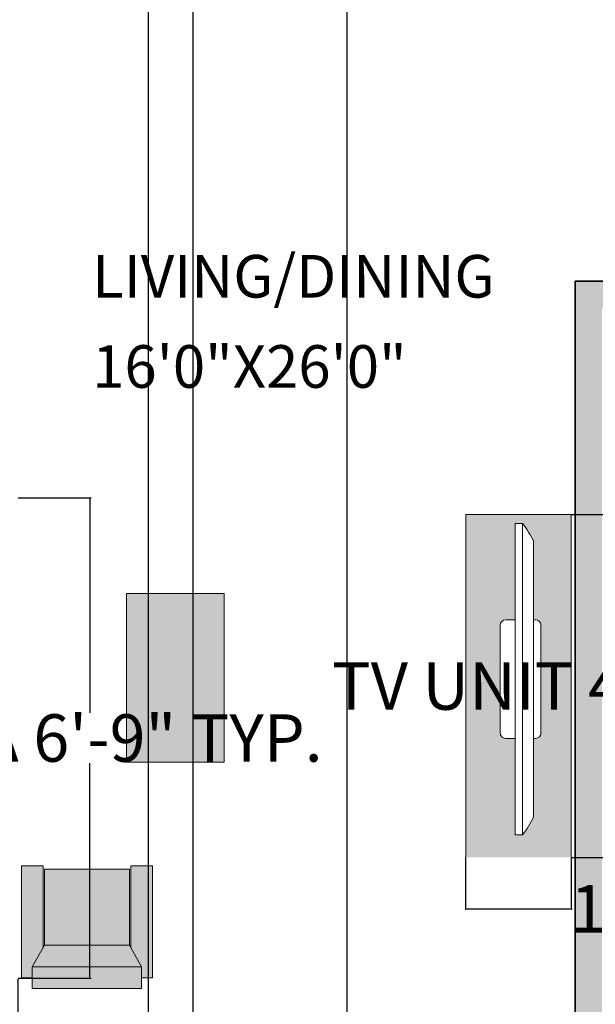
# Model space of a CAD drawing. Units: inches. Extents: x 853 to 1550, y 485 to 1596.
# Tile 6 of 18: x 1170 to 1267, y 867 to 1034. Entities that reach past the tile are written whole.
import ezdxf

# ---------------------------------------------------------------- set-up
doc = ezdxf.new("R2010")
doc.units = ezdxf.units.IN
doc.header["$MEASUREMENT"] = 0
for name, color, linetype, lineweight in [('A-ANNO-DIMS', 2, 'Continuous', 18), ('A-AREA-IDEN', 250, 'Continuous', 18), ('A-WALL-PATT', 250, 'Continuous', 13), ('furniture', 250, 'Continuous', 18), ('walls', 250, 'Continuous', 35)]:
    doc.layers.add(name, color=color, linetype=linetype, lineweight=lineweight)
doc.layers.add('A-FURN-PATT', color=254, linetype='Continuous', lineweight=13, true_color=0xfeeab9)
doc.styles.get("Standard").update_dxf_attribs({"font": 'arial.ttf'})
doc.dimstyles.get("Standard").update_dxf_attribs({"dimtxt": 8, "dimasz": 0.18, "dimexe": 0.18, "dimexo": 0.0625, "dimgap": 0.09, "dimtad": 0, "dimtih": 1, "dimtoh": 1, "dimzin": 0, "dimdsep": 46, "dimlunit": 3, "dimtxsty": 'Standard', "dimcen": 0.09, "dimadec": 0, "dimazin": 0, "dimtfac": 1, "dimtofl": 0, "dimtmove": 0, "dimatfit": 3, "dimfxl": 1, "dimtolj": 1, "dimtzin": 0, "dimarcsym": 0})

# ---------------------------------------------------------------- blocks, each defined once
blk = doc.blocks.new('FABRIC SOFA 1S')
at = {"layer": 'furniture'}
for p, q in [((3, 18.12), (34, 18.12)), ((3, 15.12), (3, 18.12)), ((34, 12.12), (34, 18.12)), ((0, -15.12), (0, 15.12)), ((6, 15.12), (0, 15.12)), ((6, -15.12), (6, 15.12)), ((12, 11.75), (6, 15.12)), ((11.33, 12.12), (34, 12.12)), ((6, -15.12), (12, -11.75)), ((11.33, -12.12), (34, -12.12)), ((34, -12.12), (34, -18.12)), ((6, -15.12), (0, -15.12)), ((3, -18.12), (3, -15.12)), ((3, -18.12), (34, -18.12))]:
    blk.add_line(p, q, dxfattribs=at)
blk.add_lwpolyline([(12, -11.75), (12, 11.75), (33, 11.75), (33, -11.75)], close=True, dxfattribs=at)
blk = doc.blocks.new('PLASMA-LARGE')
at = {"layer": 'furniture'}
for p, q in [((-7.26, 0), (7.26, 0)), ((-18.61, -1), (18.61, -1)), ((-8, -1), (-8, -0.74)), ((8, -1), (8, -0.74)), ((-21, -2.5), (21, -2.5)), ((-21, -2.5), (-21, -3.5)), ((21, -2.5), (21, -3.5)), ((-21, -3.5), (21, -3.5)), ((-8, -3.5), (-8, -4.76)), ((8, -3.5), (8, -4.76)), ((-7.26, -5.5), (7.26, -5.5))]:
    blk.add_line(p, q, dxfattribs=at)
for centre, radius, start, end in [((-7.26, -0.74), 0.744, 90, 180), ((7.26, -0.74), 0.744, 0, 90), ((-13.97, -11.05), 11.07, 114.7602, 129.4175), ((13.97, -11.05), 11.07, 50.5825, 65.2398), ((-7.26, -4.76), 0.744, 180, 270), ((7.26, -4.76), 0.744, 270, 0)]:
    blk.add_arc(centre, radius, start, end, dxfattribs=at)
blk = doc.blocks.new('TV-CONSOLE')
for p, q in [((0, 0), (0, 57.83)), ((0, 57.83), (17.81, 57.83)), ((17.81, 57.83), (17.81, 0))]:
    blk.add_line(p, q)
at = {"xscale": 1.249763490704796, "yscale": 1.249763490704796, "zscale": 1.249763490704796, "rotation": 270}
blk.add_blockref('PLASMA-LARGE', (12.71, 30.08), dxfattribs=at)
blk = doc.blocks.new('*D42')
at = {"layer": 'A-ANNO-DIMS', "color": 0, "lineweight": -2, "transparency": 16777216}
for p, q in [((1293.75, 863.63), (1282.92, 863.63)), ((1283.1, 863.45), (1283.1, 863.3)), ((1293.75, 854.63), (1282.92, 854.63)), ((1283.1, 854.81), (1283.1, 854.95))]:
    blk.add_line(p, q, dxfattribs=at)
at = {"layer": 'A-ANNO-DIMS', "color": 0, "transparency": 16777216}
for points in [[(1283.07, 863.45), (1283.13, 863.45), (1283.1, 863.63)], [(1283.07, 854.81), (1283.13, 854.81), (1283.1, 854.63)]]:
    blk.add_solid(points, dxfattribs=at)
at = {"layer": 'Defpoints', "color": 0, "transparency": 16777216}
for p in [(1283.1, 863.63), (1293.81, 863.63), (1293.81, 854.63)]:
    blk.add_point(p, dxfattribs=at)
at = {"layer": 'A-ANNO-DIMS', "color": 0, "transparency": 16777216, "insert": (1283.1, 859.13), "char_height": 8, "attachment_point": 5}
blk.add_mtext('\\A1;0\'-9" TYP.', dxfattribs=at)
blk = doc.blocks.new('*D45')
at = {"layer": 'A-ANNO-DIMS', "color": 0, "lineweight": -2, "transparency": 16777216}
for p, q in [((1263.33, 950.07), (1272.12, 950.07)), ((1271.94, 949.89), (1271.94, 925.33)), ((1271.94, 892.42), (1271.94, 916.98)), ((1263.33, 892.24), (1272.12, 892.24))]:
    blk.add_line(p, q, dxfattribs=at)
at = {"layer": 'A-ANNO-DIMS', "color": 0, "transparency": 16777216}
for points in [[(1271.91, 949.89), (1271.97, 949.89), (1271.94, 950.07)], [(1271.91, 892.42), (1271.97, 892.42), (1271.94, 892.24)]]:
    blk.add_solid(points, dxfattribs=at)
at = {"layer": 'Defpoints', "color": 0, "transparency": 16777216}
for p in [(1263.27, 950.07), (1271.94, 950.07), (1263.27, 892.24)]:
    blk.add_point(p, dxfattribs=at)
at = {"layer": 'A-ANNO-DIMS', "color": 0, "transparency": 16777216, "insert": (1271.94, 921.15), "char_height": 8, "attachment_point": 5}
blk.add_mtext('\\A1;TV UNIT 4\'-10" TYP.', dxfattribs=at)
blk = doc.blocks.new('*D46')
at = {"layer": 'A-ANNO-DIMS', "color": 0, "lineweight": -2, "transparency": 16777216}
for p, q in [((1245.45, 892.17), (1245.45, 883.38)), ((1263.27, 892.17), (1263.27, 883.38)), ((1245.63, 883.56), (1263.09, 883.56)), ((1263.27, 883.56), (1263.45, 883.56))]:
    blk.add_line(p, q, dxfattribs=at)
at = {"layer": 'A-ANNO-DIMS', "color": 0, "transparency": 16777216}
for points in [[(1245.63, 883.59), (1245.63, 883.53), (1245.45, 883.56)], [(1263.09, 883.59), (1263.09, 883.53), (1263.27, 883.56)]]:
    blk.add_solid(points, dxfattribs=at)
at = {"layer": 'Defpoints', "color": 0, "transparency": 16777216}
for p in [(1245.45, 892.24), (1263.27, 892.24), (1263.27, 883.56)]:
    blk.add_point(p, dxfattribs=at)
at = {"layer": 'A-ANNO-DIMS', "color": 0, "transparency": 16777216, "insert": (1287.54, 883.56), "char_height": 8, "attachment_point": 5}
blk.add_mtext('\\A1;1\'-6" TYP.', dxfattribs=at)
blk = doc.blocks.new('*D49')
at = {"layer": 'A-ANNO-DIMS', "color": 0, "lineweight": -2, "transparency": 16777216}
for p, q in [((1169.96, 952.92), (1182.24, 952.92)), ((1182.06, 952.74), (1182.06, 916.61)), ((1182.06, 872.02), (1182.06, 908.15)), ((1169.96, 871.84), (1182.24, 871.84))]:
    blk.add_line(p, q, dxfattribs=at)
at = {"layer": 'A-ANNO-DIMS', "color": 0, "transparency": 16777216}
for points in [[(1182.03, 952.74), (1182.09, 952.74), (1182.06, 952.92)], [(1182.03, 872.02), (1182.09, 872.02), (1182.06, 871.84)]]:
    blk.add_solid(points, dxfattribs=at)
at = {"layer": 'Defpoints', "color": 0, "transparency": 16777216}
for p in [(1169.9, 952.92), (1182.06, 952.92), (1169.9, 871.84)]:
    blk.add_point(p, dxfattribs=at)
at = {"layer": 'A-ANNO-DIMS', "color": 0, "transparency": 16777216, "insert": (1182.06, 912.38), "char_height": 8, "attachment_point": 5}
blk.add_mtext('\\A1;SOFA 6\'-9" TYP.', dxfattribs=at)
blk = doc.blocks.new('*D50')
at = {"layer": 'A-ANNO-DIMS', "color": 0, "lineweight": -2, "transparency": 16777216}
for p, q in [((1144.37, 871.78), (1144.37, 859.5)), ((1169.9, 871.78), (1169.9, 859.5)), ((1144.55, 859.68), (1169.72, 859.68)), ((1169.9, 859.68), (1170.08, 859.68))]:
    blk.add_line(p, q, dxfattribs=at)
at = {"layer": 'A-ANNO-DIMS', "color": 0, "transparency": 16777216}
for points in [[(1144.55, 859.71), (1144.55, 859.65), (1144.37, 859.68)], [(1169.72, 859.71), (1169.72, 859.65), (1169.9, 859.68)]]:
    blk.add_solid(points, dxfattribs=at)
at = {"layer": 'Defpoints', "color": 0, "transparency": 16777216}
for p in [(1144.37, 871.84), (1169.9, 871.84), (1169.9, 859.68)]:
    blk.add_point(p, dxfattribs=at)
at = {"layer": 'A-ANNO-DIMS', "color": 0, "transparency": 16777216, "insert": (1203.94, 859.68), "char_height": 8, "attachment_point": 5}
blk.add_mtext('\\A1;2\'-1 1/2" TYP.', dxfattribs=at)
blk = doc.blocks.new('*D72')
at = {"layer": 'A-ANNO-DIMS', "color": 0, "lineweight": -2, "transparency": 16777216}
for p, q in [((1139.44, 1321.07), (1139.44, 497.1)), ((1199.44, 1321.07), (1199.44, 497.1)), ((1139.62, 497.28), (1158.71, 497.28)), ((1199.26, 497.28), (1180.16, 497.28))]:
    blk.add_line(p, q, dxfattribs=at)
at = {"layer": 'A-ANNO-DIMS', "color": 0, "transparency": 16777216}
for points in [[(1139.62, 497.31), (1139.62, 497.25), (1139.44, 497.28)], [(1199.26, 497.31), (1199.26, 497.25), (1199.44, 497.28)]]:
    blk.add_solid(points, dxfattribs=at)
at = {"layer": 'Defpoints', "color": 0, "transparency": 16777216}
for p in [(1139.44, 1321.13), (1199.44, 1321.13), (1199.44, 497.28)]:
    blk.add_point(p, dxfattribs=at)
at = {"layer": 'A-ANNO-DIMS', "color": 0, "transparency": 16777216, "insert": (1169.44, 497.28), "char_height": 8, "attachment_point": 5}
blk.add_mtext('\\A1;5\'-0"', dxfattribs=at)
blk = doc.blocks.new('*D81')
at = {"layer": 'A-ANNO-DIMS', "color": 0, "lineweight": -2, "transparency": 16777216}
for p, q in [((1191.94, 767.69), (1191.94, 1584.65)), ((1225.45, 767.69), (1225.45, 1584.65)), ((1192.12, 1584.47), (1225.27, 1584.47)), ((1225.45, 1584.47), (1225.63, 1584.47))]:
    blk.add_line(p, q, dxfattribs=at)
at = {"layer": 'A-ANNO-DIMS', "color": 0, "transparency": 16777216}
for points in [[(1192.12, 1584.5), (1192.12, 1584.44), (1191.94, 1584.47)], [(1225.27, 1584.5), (1225.27, 1584.44), (1225.45, 1584.47)]]:
    blk.add_solid(points, dxfattribs=at)
at = {"layer": 'Defpoints', "color": 0, "transparency": 16777216}
for p in [(1225.45, 1584.47), (1191.94, 767.63), (1225.45, 767.63)]:
    blk.add_point(p, dxfattribs=at)
at = {"layer": 'A-ANNO-DIMS', "color": 0, "transparency": 16777216, "insert": (1245.74, 1584.47), "char_height": 8, "attachment_point": 5}
blk.add_mtext('\\A1;2\'-9 1/2"', dxfattribs=at)

msp = doc.modelspace()

# ---------------------------------------------------------------- hatches: boundary and pattern name
at = {"layer": 'A-FURN-PATT'}
h = msp.add_hatch(color=256, dxfattribs=at)
h.dxf.hatch_style = 1
h.paths.add_polyline_path([(1245.455, 950.07), (1245.455, 892.236), (1263.267, 892.236), (1263.267, 950.07)])
h.paths.add_polyline_path([(1251.288, 931.389, -0.4142136), (1252.218, 932.319), (1253.787, 932.319), (1253.787, 948.566), (1255.037, 948.566, -0.0640419), (1256.911, 945.576), (1256.911, 932.319), (1257.231, 932.319, -0.4142136), (1258.161, 931.389), (1258.161, 913.253, -0.4142136), (1257.231, 912.323), (1256.911, 912.323), (1256.911, 899.065, -0.0640419), (1255.037, 896.076), (1253.787, 896.076), (1253.787, 912.323), (1252.218, 912.323, -0.4142136), (1251.288, 913.253)], flags=16)
h = msp.add_hatch(color=256, dxfattribs=at)
h.dxf.hatch_style = 1
h.paths.add_polyline_path([(1204.713, 936.786), (1188.197, 936.786), (1188.197, 908.331), (1204.713, 908.331)])
h = msp.add_hatch(color=256, dxfattribs=at)
h.dxf.hatch_style = 1
h.paths.add_polyline_path([(1174.383, 877.43), (1174.383, 890.228), (1188.705, 890.228), (1188.705, 877.43)])
h.paths.add_polyline_path([(1172.327, 873.774), (1172.327, 871.946), (1170.498, 871.946), (1170.498, 890.838), (1174.155, 890.838), (1174.155, 877.024)])
h.paths.add_polyline_path([(1172.327, 873.774), (1174.383, 877.43), (1188.705, 877.43), (1190.762, 873.774)])
h.paths.add_polyline_path([(1172.327, 870.117), (1172.327, 873.774), (1190.762, 873.774), (1190.762, 870.117)])
h.paths.add_polyline_path([(1188.934, 877.024), (1188.934, 890.838), (1192.59, 890.838), (1192.59, 871.946), (1190.762, 871.946), (1190.762, 873.774)])
at = {"layer": 'A-WALL-PATT'}
h = msp.add_hatch(color=256, dxfattribs=at)
h.dxf.hatch_style = 1
h.paths.add_polyline_path([(990.937, 1111.29), (981.937, 1111.29), (981.937, 1044.136), (984.946, 1044.136), (990.937, 1044.136), (990.937, 1072.129), (1045.609, 1072.129, -0.0272078), (1045.453, 1074.983), (1045.453, 1076.629), (990.937, 1076.629)], flags=17)
h.paths.add_polyline_path([(1091.437, 1072.129), (1139.437, 1072.129), (1139.437, 1206.521), (1134.937, 1206.521), (1134.937, 1076.629), (1071.734, 1076.629), (1071.734, 1074.983), (1071.734, 1072.129), (1086.937, 1072.129), (1086.937, 1012.129), (990.937, 1012.129), (981.937, 1012.129), (981.937, 944.409), (990.937, 944.409), (990.937, 1007.629), (1091.437, 1007.629)])
h.paths.add_polyline_path([(990.937, 872.981), (981.937, 872.981), (981.937, 788.629), (990.937, 788.629)])
h.paths.add_polyline_path([(1014.605, 800.886), (990.937, 800.886), (990.937, 796.386), (1014.605, 796.386)])
h.paths.add_polyline_path([(1134.937, 793.129), (1090.727, 793.129), (1090.727, 788.629), (1134.937, 788.629)])
h.paths.add_polyline_path([(1139.437, 800.892), (1134.937, 800.892), (1134.937, 788.629), (1113.94, 788.629), (1113.94, 767.629), (1139.437, 767.629), (1191.938, 767.629), (1191.938, 772.657), (1191.938, 776.629), (1139.437, 776.629)])
h.paths.add_polyline_path([(1131.331, 781.621), (1131.331, 775.236), (1118.809, 775.236), (1118.809, 781.621)], flags=16)
h.paths.add_polyline_path([(1131.331, 781.621), (1118.809, 781.621), (1118.809, 775.236), (1131.331, 775.236)], flags=0)
h.paths.add_polyline_path([(1118.963, 707.356), (1110.94, 707.356), (1110.94, 699.868), (1118.963, 699.868)])
h.paths.add_polyline_path([(1284.919, 707.356), (1276.896, 707.356), (1276.896, 699.868), (1284.919, 699.868)])
h.paths.add_polyline_path([(1293.812, 863.629), (1268.437, 863.629), (1268.437, 984.936), (1308.937, 984.936), (1308.937, 996.627), (1304.437, 996.627), (1304.437, 989.436), (1263.937, 989.436), (1263.937, 863.629), (1215.364, 863.629), (1215.364, 854.629), (1252.179, 854.629), (1252.179, 776.629), (1225.216, 776.629, -0.0297134), (1225.453, 772.657), (1225.453, 767.629), (1261.179, 767.629), (1261.179, 854.629), (1293.812, 854.629)])
h.paths.add_polyline_path([(1176.151, 863.629), (1139.437, 863.629), (1139.437, 854.629), (1176.151, 854.629)])
h.paths.add_polyline_path([(1134.937, 863.629), (1109.834, 863.629), (1109.834, 859.129), (1134.937, 859.129)])
h.paths.add_polyline_path([(1148.879, 950.672), (1144.374, 950.672), (1144.374, 874.094), (1148.879, 874.094)])
h.paths.add_polyline_path([(1079.778, 863.629), (990.937, 863.629), (990.937, 859.129), (1079.778, 859.129)])

# ---------------------------------------------------------------- linework, layer by layer
at = {"layer": 'furniture'}
for p, q in [((1188.197, 936.786), (1204.713, 936.786)), ((1188.197, 908.331), (1188.197, 936.786)), ((1204.713, 936.786), (1204.713, 908.331)), ((1204.713, 908.331), (1188.197, 908.331))]:
    msp.add_line(p, q, dxfattribs=at)
at = {"layer": 'walls'}
for p, q in [((1263.937, 863.629), (1263.937, 989.436)), ((1263.937, 989.436), (1304.437, 989.436))]:
    msp.add_line(p, q, dxfattribs=at)

# ---------------------------------------------------------------- block references
at = {"layer": 'furniture'}
msp.add_blockref('TV-CONSOLE', (1245.455, 892.236), dxfattribs=at)
at = {"layer": 'furniture', "xscale": 0.6094251026746103, "yscale": 0.6094251026746103, "zscale": 0.6094251026746103, "rotation": 90}
msp.add_blockref('FABRIC SOFA 1S', (1181.544, 870.117), dxfattribs=at)

# ---------------------------------------------------------------- texts
at = {"layer": 'A-AREA-IDEN'}
for s, p in [('LIVING/DINING', (1182.426, 986.678)), ('16\'0"X26\'0"', (1182.426, 971.459))]:
    msp.add_text(s, height=7.19435, dxfattribs=at).set_placement(p)

# ---------------------------------------------------------------- dimensions: what is measured, and where the dimension line sits
at = {"layer": 'A-ANNO-DIMS'}
for base, p1, p2, picture, middle in [((1225.453, 1584.468), (1191.938, 767.629), (1225.453, 767.629), '*D81', (1245.744, 1584.468)), ((1199.437, 497.279), (1139.437, 1321.129), (1199.437, 1321.129), '*D72', (1169.437, 497.279))]:
    dim = msp.add_linear_dim(base=base, p1=p1, p2=p2, dimstyle='Standard', override={"dimdec": 1, "dimlfac": 1, "dimrnd": 0, "dimzin": 1, "dimdsep": 46, "dimlunit": 4, "dimfrac": 2}, dxfattribs=at)
    dim.commit()
    dim.dimension.update_dxf_attribs({"geometry": picture, "text_midpoint": middle})
for base, p1, p2, text, picture, middle in [((1182.062, 952.924), (1169.9, 871.842), (1169.9, 952.924), 'SOFA <> TYP.', '*D49', (1182.062, 912.383)), ((1271.942, 950.07), (1263.267, 892.236), (1263.267, 950.07), 'TV UNIT <> TYP.', '*D45', (1271.942, 921.153)), ((1283.098, 863.629), (1293.812, 854.629), (1293.812, 863.629), '<> TYP.', '*D42', (1283.098, 859.129))]:
    dim = msp.add_linear_dim(base=base, p1=p1, p2=p2, angle=90, text=text, dimstyle='Standard', override={"dimdec": 1, "dimlfac": 1, "dimrnd": 0, "dimzin": 1, "dimdsep": 46, "dimlunit": 4, "dimfrac": 2}, dxfattribs=at)
    dim.commit()
    dim.dimension.update_dxf_attribs({"geometry": picture, "text_midpoint": middle})
for base, p1, p2, picture, middle in [((1263.267, 883.561), (1245.455, 892.236), (1263.267, 892.236), '*D46', (1287.542, 883.561)), ((1169.9, 859.68), (1144.374, 871.842), (1169.9, 871.842), '*D50', (1203.941, 859.68))]:
    dim = msp.add_linear_dim(base=base, p1=p1, p2=p2, text='<> TYP.', dimstyle='Standard', override={"dimdec": 1, "dimlfac": 1, "dimrnd": 0, "dimzin": 1, "dimdsep": 46, "dimlunit": 4, "dimfrac": 2}, dxfattribs=at)
    dim.commit()
    dim.dimension.update_dxf_attribs({"geometry": picture, "text_midpoint": middle})

doc.saveas('drawing.dxf')
